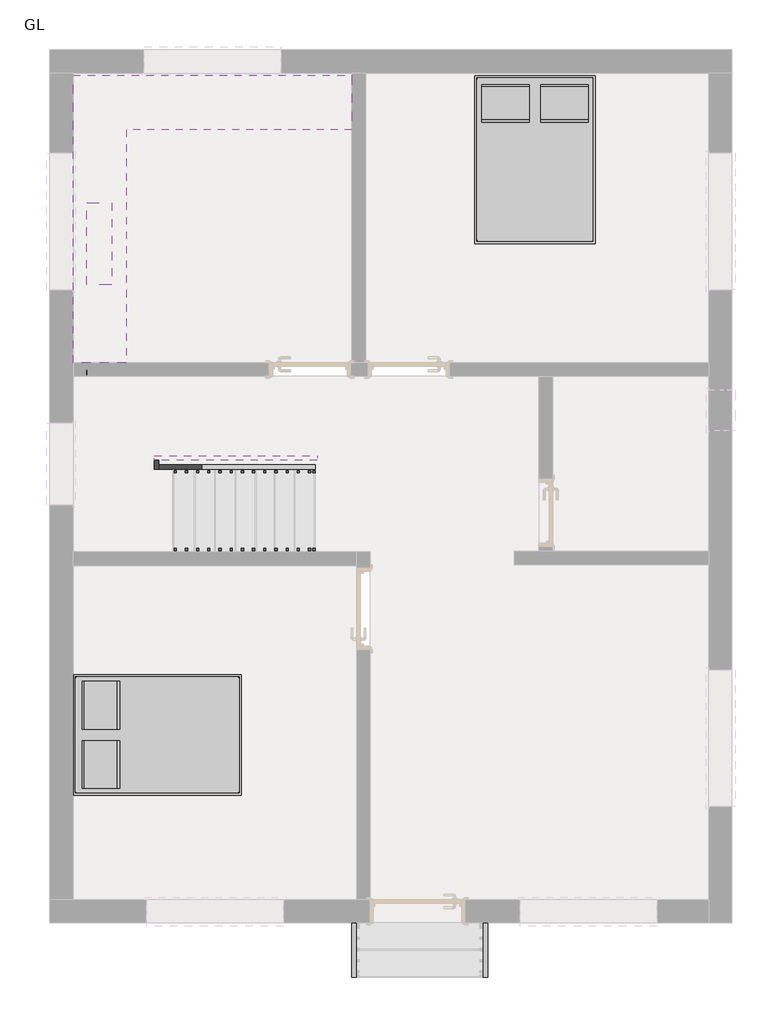
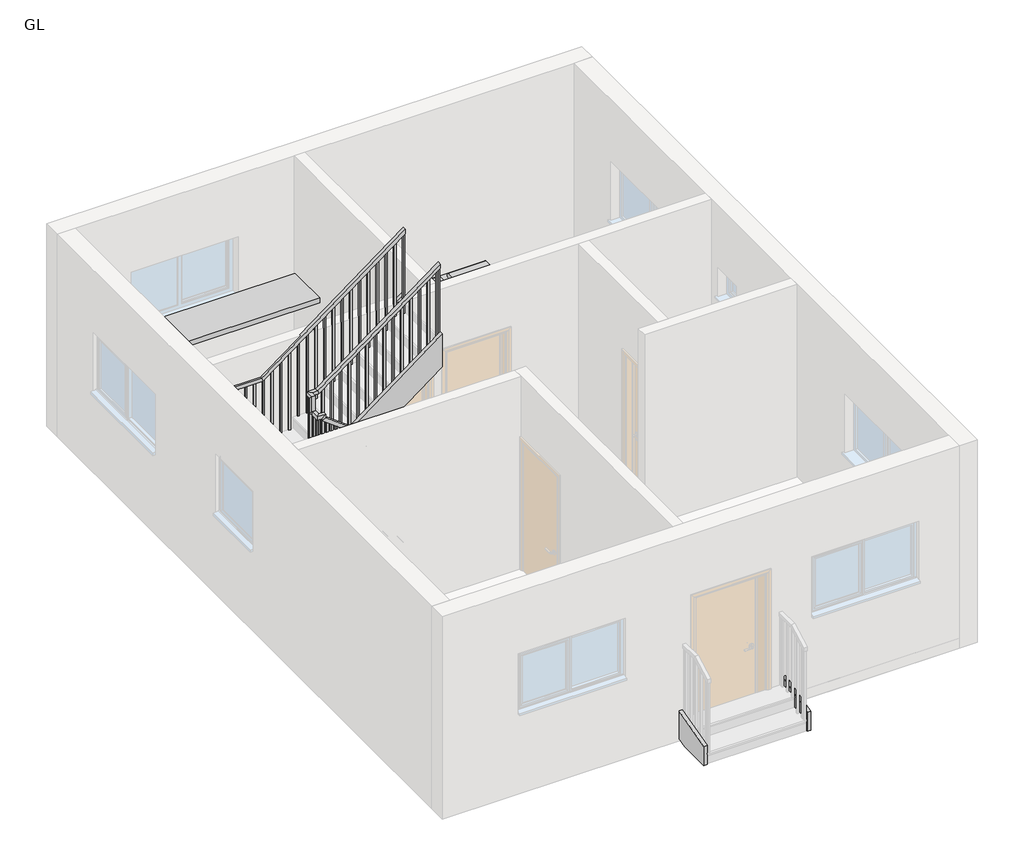
# One storey, part 2 of 2: 8 members, 2 furniture elements, 2 proxies, 2 railings.
"""IFC4 building model written with IfcOpenShell, lengths in millimetres."""

from ifc_helpers import new_model, si_unit, frame, origin, place, context, project, spatial, polyline, outline, extrude, faceted_brep, transform, mapped, element, save
from components import generic_models_1_generic_models_1_ec2a76fc, generic_models_2_generic_models_2_056d5301, furniture_bed_1_1346x1880x355mm_double_93dec6ea

model = new_model("IFC4")

# Units and contexts
model_context = context("Model", 3, world=origin())
ifc_project = project(units=[si_unit("LENGTHUNIT", "METRE", prefix="MILLI")], contexts=[model_context])

# Site, building, storey
site = spatial("IfcSite", under=ifc_project)
building = spatial("IfcBuilding", under=site)
storey = spatial("IfcBuildingStorey", under=building, Name="GL", Elevation=0.0)

# Proxies
placement = place(None, origin())
generic_models_1_generic_models_1_shape = generic_models_1_generic_models_1_ec2a76fc(model_context)
element("IfcBuildingElementProxy", 1, Name="Generic Models 1 : Generic Models 1", ObjectType="Generic Models 1 : Generic Models 1", at=placement, inside=storey, context=model_context, shape_type="MappedRepresentation", body=[
    mapped(generic_models_1_generic_models_1_shape, transform((0.0, 0.0, 0.0), x_axis=(1.0, 0.0, 0.0), y_axis=(0.0, 1.0, 0.0), z_axis=(0.0, 0.0, 1.0))),
])
generic_models_2_generic_models_2_shape = generic_models_2_generic_models_2_056d5301(model_context)
element("IfcBuildingElementProxy", 2, Name="Generic Models 2 : Generic Models 2", ObjectType="Generic Models 2 : Generic Models 2", at=placement, inside=storey, context=model_context, shape_type="MappedRepresentation", body=[
    mapped(generic_models_2_generic_models_2_shape, transform((0.0, 0.0, 0.0), x_axis=(1.0, 0.0, 0.0), y_axis=(0.0, 1.0, 0.0), z_axis=(0.0, 0.0, 1.0))),
])

# Furniture
furniture_bed_1_1346x1880x355mm_double_shape = furniture_bed_1_1346x1880x355mm_double_93dec6ea(model_context)
element("IfcFurniture", 3, ObjectType="Furniture_Bed_1 : 1346x1880x355mm-Double", at=placement, inside=storey, context=model_context, shape_type="MappedRepresentation", body=[
    mapped(furniture_bed_1_1346x1880x355mm_double_shape, transform((6044.9756135, 10437.9267123, 149.9616), x_axis=(1.0, 0.0, 0.0), y_axis=(0.0, 1.0, 0.0), z_axis=(0.0, 0.0, 1.0))),
])
element("IfcFurniture", 4, ObjectType="Furniture_Bed_1 : 1346x1880x355mm-Double", at=placement, inside=storey, context=model_context, shape_type="MappedRepresentation", body=[
    mapped(furniture_bed_1_1346x1880x355mm_double_shape, transform((1929.3384143, 3437.1747451, 149.9616), x_axis=(0.0, 1.0, 0.0), y_axis=(-1.0, 0.0, 0.0), z_axis=(0.0, 0.0, 1.0))),
])

# Members
element("IfcMember", 5, ObjectType="Stringer-50mm_Width", at=placement, inside=storey, context=model_context, shape_type="SweptSolid", body=[
    extrude(outline(polyline([(0.0, 3927.9747157), (240.3799463, 3927.9747157), (1566.4365081, 2174.3169781), (1566.4365081, 1511.1244088), (0.0, 3582.6751873), (0.0, 3927.9747157)])), frame((0.0, 5770.9272041, 0.0), z_axis=(0.0, 1.0, 0.0), x_axis=(0.0, 0.0, 1.0)), (0.0, 0.0, 1.0), 50.0),
])
element("IfcMember", 6, ObjectType="Stringer-50mm_Width", at=placement, inside=storey, context=model_context, shape_type="SweptSolid", body=[
    extrude(outline(polyline([(1223.7679225, 5770.9272041), (1173.7679225, 5770.9272041), (1173.7679225, 7802.1353898), (1223.7679225, 7802.1353898), (1223.7679225, 5770.9272041)])), frame((0.0, 0.0, 1166.4365081), z_axis=(0.0, 0.0, 1.0), x_axis=(1.0, 0.0, 0.0)), (0.0, 0.0, 1.0), 400.0),
])
element("IfcMember", 7, ObjectType="Stringer-50mm_Width", at=placement, inside=storey, context=model_context, shape_type="SweptSolid", body=[
    extrude(outline(polyline([(1166.4365081, 1997.5960405), (2630.7773804, 3949.8187157), (3130.7987558, 3949.8187157), (1166.4365081, 1330.9800323), (1166.4365081, 1997.5960405)])), frame((0.0, 7802.1353898, 0.0), z_axis=(0.0, 1.0, 0.0), x_axis=(0.0, 0.0, 1.0)), (0.0, 0.0, 1.0), 50.0),
])
element("IfcMember", 8, ObjectType="Stringer-50mm_Width", at=placement, inside=storey, context=model_context, shape_type="SweptSolid", body=[
    extrude(outline(polyline([(0.0, 3927.9747157), (240.3799463, 3927.9747157), (1560.7645481, 2181.8179225), (1059.2807982, 2181.8179225), (0.0, 3582.6751873), (0.0, 3927.9747157)])), frame((0.0, 6741.6853898, 0.0), z_axis=(0.0, 1.0, 0.0), x_axis=(0.0, 0.0, 1.0)), (0.0, 0.0, 1.0), 50.0),
])
element("IfcMember", 9, ObjectType="Stringer-50mm_Width", at=placement, inside=storey, context=model_context, shape_type="SweptSolid", body=[
    extrude(outline(polyline([(2181.8179225, 6741.6853898), (2131.8179225, 6741.6853898), (2131.8179225, 6844.0853898), (2181.8179225, 6844.0853898), (2181.8179225, 6741.6853898)])), frame((0.0, 0.0, 1166.4365081), z_axis=(0.0, 0.0, 1.0), x_axis=(1.0, 0.0, 0.0)), (0.0, 0.0, 1.0), 400.0),
])
element("IfcMember", 10, ObjectType="Stringer-50mm_Width", at=placement, inside=storey, context=model_context, shape_type="SweptSolid", body=[
    extrude(outline(polyline([(1767.1362488, 2131.8179225), (1267.1148735, 2131.8179225), (2630.7773804, 3949.8187157), (3130.7987558, 3949.8187157), (1767.1362488, 2131.8179225)])), frame((0.0, 6844.0853898, 0.0), z_axis=(0.0, 1.0, 0.0), x_axis=(0.0, 0.0, 1.0)), (0.0, 0.0, 1.0), 50.0),
])
element("IfcMember", 11, ObjectType="Stringer-50mm_Width", at=placement, inside=storey, context=model_context, shape_type="SweptSolid", body=[
    extrude(outline(polyline([(1066.0472041, 0.0), (1066.0472041, 285.8067966), (1675.6472041, 455.14013), (1675.6472041, 39.994759), (1531.6660715, 0.0), (1066.0472041, 0.0)])), frame((4335.1747157, 0.0, 0.0), z_axis=(1.0, 0.0, 0.0), x_axis=(0.0, 1.0, 0.0)), (0.0, 0.0, 1.0), 50.0),
])
element("IfcMember", 12, ObjectType="Stringer-50mm_Width", at=placement, inside=storey, context=model_context, shape_type="SweptSolid", body=[
    extrude(outline(polyline([(1066.0472041, 0.0), (1066.0472041, 285.8067966), (1675.6472041, 455.14013), (1675.6472041, 39.994759), (1531.6660715, 0.0), (1066.0472041, 0.0)])), frame((5807.5747157, 0.0, 0.0), z_axis=(1.0, 0.0, 0.0), x_axis=(0.0, 1.0, 0.0)), (0.0, 0.0, 1.0), 50.0),
])

# Railings
element("IfcRailing", 13, ObjectType="1100mm", at=placement, inside=storey, context=model_context, shape_type="SolidModel", body=[
    faceted_brep([(3927.9747157, 6691.2853898, 1269.3333333), (3927.9747157, 6691.2853898, 1206.7070206), (3927.9747157, 6741.2853898, 1206.7070206), (3927.9747157, 6741.2853898, 1269.3333333), (2206.4179225, 6691.2853898, 2567.7364635), (2156.4179225, 6691.2853898, 2542.8202959), (2156.4179225, 6741.2853898, 2542.8202959), (2206.4179225, 6741.2853898, 2567.7364635), (2206.4179225, 6691.2853898, 2624.0), (2156.4179225, 6691.2853898, 2574.0), (2156.4179225, 6741.2853898, 2574.0), (2206.4179225, 6741.2853898, 2624.0), (2081.4179225, 6691.2853898, 2624.0), (2081.4179225, 6691.2853898, 2574.0), (2131.4179225, 6741.2853898, 2574.0), (2131.4179225, 6741.2853898, 2624.0), (2081.4179225, 6816.2853898, 2624.0), (2081.4179225, 6816.2853898, 2574.0), (2131.4179225, 6816.2853898, 2574.0), (2131.4179225, 6816.2853898, 2624.0), (2081.4179225, 6819.4853898, 2624.0), (2081.4179225, 6869.4853898, 2574.0), (2131.4179225, 6869.4853898, 2574.0), (2131.4179225, 6819.4853898, 2624.0), (2081.4179225, 6819.4853898, 2848.9208412), (2081.4179225, 6869.4853898, 2798.9208412), (2131.4179225, 6869.4853898, 2798.9208412), (2131.4179225, 6819.4853898, 2848.9208412), (2081.4179225, 6944.4853898, 2848.9208412), (2081.4179225, 6944.4853898, 2798.9208412), (2131.4179225, 6894.4853898, 2798.9208412), (2131.4179225, 6894.4853898, 2848.9208412), (2206.4179225, 6944.4853898, 2848.9208412), (2222.9980476, 6944.4853898, 2798.9208412), (2222.9980476, 6894.4853898, 2798.9208412), (2206.4179225, 6894.4853898, 2848.9208412), (3949.8187157, 6944.4853898, 4148.0), (3949.8187157, 6894.4853898, 4148.0), (3949.8187157, 6894.4853898, 4085.6454714), (3949.8187157, 6944.4853898, 4085.6454714)], [[[0, 1, 2, 3]], [[1, 0, 4, 5]], [[2, 1, 5, 6]], [[3, 2, 6, 7]], [[0, 3, 7, 4]], [[5, 4, 8, 9]], [[6, 5, 9, 10]], [[7, 6, 10, 11]], [[4, 7, 11, 8]], [[9, 8, 12, 13]], [[10, 9, 13, 14]], [[11, 10, 14, 15]], [[8, 11, 15, 12]], [[13, 12, 16, 17]], [[14, 13, 17, 18]], [[15, 14, 18, 19]], [[12, 15, 19, 16]], [[17, 16, 20, 21]], [[18, 17, 21, 22]], [[19, 18, 22, 23]], [[16, 19, 23, 20]], [[21, 20, 24, 25]], [[22, 21, 25, 26]], [[23, 22, 26, 27]], [[20, 23, 27, 24]], [[25, 24, 28, 29]], [[26, 25, 29, 30]], [[27, 26, 30, 31]], [[24, 27, 31, 28]], [[29, 28, 32, 33]], [[30, 29, 33, 34]], [[31, 30, 34, 35]], [[28, 31, 35, 32]], [[36, 37, 38, 39]], [[33, 32, 36, 39]], [[34, 33, 39, 38]], [[35, 34, 38, 37]], [[32, 35, 37, 36]]]),
    extrude(outline(polyline([(4053.3057673, 3906.4179225), (2878.6666667, 3906.4179225), (2878.6666667, 3931.4179225), (4071.9342886, 3931.4179225), (4053.3057673, 3906.4179225)])), frame((0.0, 6906.9853898, 0.0), z_axis=(0.0, 1.0, 0.0), x_axis=(0.0, 0.0, 1.0)), (0.0, 0.0, 1.0), 25.0),
    extrude(outline(polyline([(3960.1631603, 3781.4179225), (2878.6666667, 3781.4179225), (2878.6666667, 3806.4179225), (3978.7916817, 3806.4179225), (3960.1631603, 3781.4179225)])), frame((0.0, 6906.9853898, 0.0), z_axis=(0.0, 1.0, 0.0), x_axis=(0.0, 0.0, 1.0)), (0.0, 0.0, 1.0), 25.0),
    extrude(outline(polyline([(3867.0205533, 3656.4179225), (2709.3333333, 3656.4179225), (2709.3333333, 3681.4179225), (3885.6490747, 3681.4179225), (3867.0205533, 3656.4179225)])), frame((0.0, 6906.9853898, 0.0), z_axis=(0.0, 1.0, 0.0), x_axis=(0.0, 0.0, 1.0)), (0.0, 0.0, 1.0), 25.0),
    extrude(outline(polyline([(3773.8779464, 3531.4179225), (2709.3333333, 3531.4179225), (2709.3333333, 3556.4179225), (3792.5064678, 3556.4179225), (3773.8779464, 3531.4179225)])), frame((0.0, 6906.9853898, 0.0), z_axis=(0.0, 1.0, 0.0), x_axis=(0.0, 0.0, 1.0)), (0.0, 0.0, 1.0), 25.0),
    extrude(outline(polyline([(3680.7353394, 3406.4179225), (2540.0, 3406.4179225), (2540.0, 3431.4179225), (3699.3638608, 3431.4179225), (3680.7353394, 3406.4179225)])), frame((0.0, 6906.9853898, 0.0), z_axis=(0.0, 1.0, 0.0), x_axis=(0.0, 0.0, 1.0)), (0.0, 0.0, 1.0), 25.0),
    extrude(outline(polyline([(3587.5927324, 3281.4179225), (2540.0, 3281.4179225), (2540.0, 3306.4179225), (3606.2212538, 3306.4179225), (3587.5927324, 3281.4179225)])), frame((0.0, 6906.9853898, 0.0), z_axis=(0.0, 1.0, 0.0), x_axis=(0.0, 0.0, 1.0)), (0.0, 0.0, 1.0), 25.0),
    extrude(outline(polyline([(3494.4501255, 3156.4179225), (2370.6666667, 3156.4179225), (2370.6666667, 3181.4179225), (3513.0786469, 3181.4179225), (3494.4501255, 3156.4179225)])), frame((0.0, 6906.9853898, 0.0), z_axis=(0.0, 1.0, 0.0), x_axis=(0.0, 0.0, 1.0)), (0.0, 0.0, 1.0), 25.0),
    extrude(outline(polyline([(3401.3075185, 3031.4179225), (2370.6666667, 3031.4179225), (2370.6666667, 3056.4179225), (3419.9360399, 3056.4179225), (3401.3075185, 3031.4179225)])), frame((0.0, 6906.9853898, 0.0), z_axis=(0.0, 1.0, 0.0), x_axis=(0.0, 0.0, 1.0)), (0.0, 0.0, 1.0), 25.0),
    extrude(outline(polyline([(3308.1649116, 2906.4179225), (2201.3333333, 2906.4179225), (2201.3333333, 2931.4179225), (3326.7934329, 2931.4179225), (3308.1649116, 2906.4179225)])), frame((0.0, 6906.9853898, 0.0), z_axis=(0.0, 1.0, 0.0), x_axis=(0.0, 0.0, 1.0)), (0.0, 0.0, 1.0), 25.0),
    extrude(outline(polyline([(3215.0223046, 2781.4179225), (2032.0, 2781.4179225), (2032.0, 2806.4179225), (3233.650826, 2806.4179225), (3215.0223046, 2781.4179225)])), frame((0.0, 6906.9853898, 0.0), z_axis=(0.0, 1.0, 0.0), x_axis=(0.0, 0.0, 1.0)), (0.0, 0.0, 1.0), 25.0),
    extrude(outline(polyline([(3121.8796976, 2656.4179225), (2032.0, 2656.4179225), (2032.0, 2681.4179225), (3140.508219, 2681.4179225), (3121.8796976, 2656.4179225)])), frame((0.0, 6906.9853898, 0.0), z_axis=(0.0, 1.0, 0.0), x_axis=(0.0, 0.0, 1.0)), (0.0, 0.0, 1.0), 25.0),
    extrude(outline(polyline([(3028.7370907, 2531.4179225), (1862.6666667, 2531.4179225), (1862.6666667, 2556.4179225), (3047.3656121, 2556.4179225), (3028.7370907, 2531.4179225)])), frame((0.0, 6906.9853898, 0.0), z_axis=(0.0, 1.0, 0.0), x_axis=(0.0, 0.0, 1.0)), (0.0, 0.0, 1.0), 25.0),
    extrude(outline(polyline([(2935.5944837, 2406.4179225), (1862.6666667, 2406.4179225), (1862.6666667, 2431.4179225), (2954.2230051, 2431.4179225), (2935.5944837, 2406.4179225)])), frame((0.0, 6906.9853898, 0.0), z_axis=(0.0, 1.0, 0.0), x_axis=(0.0, 0.0, 1.0)), (0.0, 0.0, 1.0), 25.0),
    extrude(outline(polyline([(2842.4518767, 2281.4179225), (1693.3333333, 2281.4179225), (1693.3333333, 2306.4179225), (2861.0803981, 2306.4179225), (2842.4518767, 2281.4179225)])), frame((0.0, 6906.9853898, 0.0), z_axis=(0.0, 1.0, 0.0), x_axis=(0.0, 0.0, 1.0)), (0.0, 0.0, 1.0), 25.0),
    extrude(outline(polyline([(2156.4179225, 6906.9853898), (2156.4179225, 6931.9853898), (2181.4179225, 6931.9853898), (2181.4179225, 6906.9853898), (2156.4179225, 6906.9853898)])), frame((0.0, 0.0, 1693.3333333), z_axis=(0.0, 0.0, 1.0), x_axis=(1.0, 0.0, 0.0)), (0.0, 0.0, 1.0), 1105.5875078),
    extrude(outline(polyline([(2118.9179225, 6891.2853898), (2093.9179225, 6891.2853898), (2093.9179225, 6916.2853898), (2118.9179225, 6916.2853898), (2118.9179225, 6891.2853898)])), frame((0.0, 0.0, 1524.0), z_axis=(0.0, 0.0, 1.0), x_axis=(1.0, 0.0, 0.0)), (0.0, 0.0, 1.0), 1274.9208412),
    extrude(outline(polyline([(2118.9179225, 6766.2853898), (2093.9179225, 6766.2853898), (2093.9179225, 6791.2853898), (2118.9179225, 6791.2853898), (2118.9179225, 6766.2853898)])), frame((0.0, 0.0, 1524.0), z_axis=(0.0, 0.0, 1.0), x_axis=(1.0, 0.0, 0.0)), (0.0, 0.0, 1.0), 1050.0),
    extrude(outline(polyline([(2127.9747157, 6728.7853898), (2127.9747157, 6703.7853898), (2102.9747157, 6703.7853898), (2102.9747157, 6728.7853898), (2127.9747157, 6728.7853898)])), frame((0.0, 0.0, 1524.0), z_axis=(0.0, 0.0, 1.0), x_axis=(1.0, 0.0, 0.0)), (0.0, 0.0, 1.0), 1050.0),
    extrude(outline(polyline([(1354.6666667, 2252.9747157), (2469.9968822, 2252.9747157), (2488.8519548, 2227.9747157), (1354.6666667, 2227.9747157), (1354.6666667, 2252.9747157)])), frame((0.0, 6703.7853898, 0.0), z_axis=(0.0, 1.0, 0.0), x_axis=(0.0, 0.0, 1.0)), (0.0, 0.0, 1.0), 25.0),
    extrude(outline(polyline([(1185.3333333, 2377.9747157), (2375.7215194, 2377.9747157), (2394.576592, 2352.9747157), (1185.3333333, 2352.9747157), (1185.3333333, 2377.9747157)])), frame((0.0, 6703.7853898, 0.0), z_axis=(0.0, 1.0, 0.0), x_axis=(0.0, 0.0, 1.0)), (0.0, 0.0, 1.0), 25.0),
    extrude(outline(polyline([(1185.3333333, 2502.9747157), (2281.4461566, 2502.9747157), (2300.3012292, 2477.9747157), (1185.3333333, 2477.9747157), (1185.3333333, 2502.9747157)])), frame((0.0, 6703.7853898, 0.0), z_axis=(0.0, 1.0, 0.0), x_axis=(0.0, 0.0, 1.0)), (0.0, 0.0, 1.0), 25.0),
    extrude(outline(polyline([(1016.0, 2627.9747157), (2187.1707938, 2627.9747157), (2206.0258664, 2602.9747157), (1016.0, 2602.9747157), (1016.0, 2627.9747157)])), frame((0.0, 6703.7853898, 0.0), z_axis=(0.0, 1.0, 0.0), x_axis=(0.0, 0.0, 1.0)), (0.0, 0.0, 1.0), 25.0),
    extrude(outline(polyline([(1016.0, 2752.9747157), (2092.895431, 2752.9747157), (2111.7505036, 2727.9747157), (1016.0, 2727.9747157), (1016.0, 2752.9747157)])), frame((0.0, 6703.7853898, 0.0), z_axis=(0.0, 1.0, 0.0), x_axis=(0.0, 0.0, 1.0)), (0.0, 0.0, 1.0), 25.0),
    extrude(outline(polyline([(846.6666667, 2877.9747157), (1998.6200682, 2877.9747157), (2017.4751408, 2852.9747157), (846.6666667, 2852.9747157), (846.6666667, 2877.9747157)])), frame((0.0, 6703.7853898, 0.0), z_axis=(0.0, 1.0, 0.0), x_axis=(0.0, 0.0, 1.0)), (0.0, 0.0, 1.0), 25.0),
    extrude(outline(polyline([(846.6666667, 3002.9747157), (1904.3447054, 3002.9747157), (1923.1997779, 2977.9747157), (846.6666667, 2977.9747157), (846.6666667, 3002.9747157)])), frame((0.0, 6703.7853898, 0.0), z_axis=(0.0, 1.0, 0.0), x_axis=(0.0, 0.0, 1.0)), (0.0, 0.0, 1.0), 25.0),
    extrude(outline(polyline([(677.3333333, 3127.9747157), (1810.0693426, 3127.9747157), (1828.9244151, 3102.9747157), (677.3333333, 3102.9747157), (677.3333333, 3127.9747157)])), frame((0.0, 6703.7853898, 0.0), z_axis=(0.0, 1.0, 0.0), x_axis=(0.0, 0.0, 1.0)), (0.0, 0.0, 1.0), 25.0),
    extrude(outline(polyline([(677.3333333, 3252.9747157), (1715.7939798, 3252.9747157), (1734.6490523, 3227.9747157), (677.3333333, 3227.9747157), (677.3333333, 3252.9747157)])), frame((0.0, 6703.7853898, 0.0), z_axis=(0.0, 1.0, 0.0), x_axis=(0.0, 0.0, 1.0)), (0.0, 0.0, 1.0), 25.0),
    extrude(outline(polyline([(508.0, 3377.9747157), (1621.518617, 3377.9747157), (1640.3736895, 3352.9747157), (508.0, 3352.9747157), (508.0, 3377.9747157)])), frame((0.0, 6703.7853898, 0.0), z_axis=(0.0, 1.0, 0.0), x_axis=(0.0, 0.0, 1.0)), (0.0, 0.0, 1.0), 25.0),
    extrude(outline(polyline([(338.6666667, 3502.9747157), (1527.2432542, 3502.9747157), (1546.0983267, 3477.9747157), (338.6666667, 3477.9747157), (338.6666667, 3502.9747157)])), frame((0.0, 6703.7853898, 0.0), z_axis=(0.0, 1.0, 0.0), x_axis=(0.0, 0.0, 1.0)), (0.0, 0.0, 1.0), 25.0),
    extrude(outline(polyline([(338.6666667, 3627.9747157), (1432.9678913, 3627.9747157), (1451.8229639, 3602.9747157), (338.6666667, 3602.9747157), (338.6666667, 3627.9747157)])), frame((0.0, 6703.7853898, 0.0), z_axis=(0.0, 1.0, 0.0), x_axis=(0.0, 0.0, 1.0)), (0.0, 0.0, 1.0), 25.0),
    extrude(outline(polyline([(169.3333333, 3752.9747157), (1338.6925285, 3752.9747157), (1357.5476011, 3727.9747157), (169.3333333, 3727.9747157), (169.3333333, 3752.9747157)])), frame((0.0, 6703.7853898, 0.0), z_axis=(0.0, 1.0, 0.0), x_axis=(0.0, 0.0, 1.0)), (0.0, 0.0, 1.0), 25.0),
    extrude(outline(polyline([(169.3333333, 3877.9747157), (1244.4171657, 3877.9747157), (1263.2722383, 3852.9747157), (169.3333333, 3852.9747157), (169.3333333, 3877.9747157)])), frame((0.0, 6703.7853898, 0.0), z_axis=(0.0, 1.0, 0.0), x_axis=(0.0, 0.0, 1.0)), (0.0, 0.0, 1.0), 25.0),
    extrude(outline(polyline([(2118.9179225, 6906.9853898), (2093.9179225, 6906.9853898), (2093.9179225, 6931.9853898), (2118.9179225, 6931.9853898), (2118.9179225, 6906.9853898)])), frame((0.0, 0.0, 1524.0), z_axis=(0.0, 0.0, 1.0), x_axis=(1.0, 0.0, 0.0)), (0.0, 0.0, 1.0), 1274.9208412),
    extrude(outline(polyline([(2118.9179225, 6728.7853898), (2118.9179225, 6703.7853898), (2093.9179225, 6703.7853898), (2093.9179225, 6728.7853898), (2118.9179225, 6728.7853898)])), frame((0.0, 0.0, 1524.0), z_axis=(0.0, 0.0, 1.0), x_axis=(1.0, 0.0, 0.0)), (0.0, 0.0, 1.0), 1050.0),
    extrude(outline(polyline([(4067.01695, 3924.8187157), (2878.6666667, 3924.8187157), (2878.6666667, 3949.8187157), (4085.6454714, 3949.8187157), (4067.01695, 3924.8187157)])), frame((0.0, 6906.9853898, 0.0), z_axis=(0.0, 1.0, 0.0), x_axis=(0.0, 0.0, 1.0)), (0.0, 0.0, 1.0), 25.0),
    extrude(outline(polyline([(169.3333333, 3927.9747157), (1206.7070206, 3927.9747157), (1225.5620932, 3902.9747157), (169.3333333, 3902.9747157), (169.3333333, 3927.9747157)])), frame((0.0, 6703.7853898, 0.0), z_axis=(0.0, 1.0, 0.0), x_axis=(0.0, 0.0, 1.0)), (0.0, 0.0, 1.0), 25.0),
])
element("IfcRailing", 14, ObjectType="1100mm", at=placement, inside=storey, context=model_context, shape_type="SolidModel", body=[
    faceted_brep([(3927.9747157, 5821.3272041, 1269.3333333), (3927.9747157, 5821.3272041, 1206.7070206), (3927.9747157, 5871.3272041, 1206.7070206), (3927.9747157, 5871.3272041, 1269.3333333), (2131.8179225, 5821.3272041, 2624.0), (2115.0766548, 5821.3272041, 2574.0), (2115.0766548, 5871.3272041, 2574.0), (2131.8179225, 5871.3272041, 2624.0), (1224.1679225, 5821.3272041, 2624.0), (1224.1679225, 5821.3272041, 2574.0), (1274.1679225, 5871.3272041, 2574.0), (1274.1679225, 5871.3272041, 2624.0), (1224.1679225, 7801.7353898, 2624.0), (1224.1679225, 7801.7353898, 2574.0), (1274.1679225, 7751.7353898, 2574.0), (1274.1679225, 7751.7353898, 2624.0), (1904.5678234, 7801.7353898, 2624.0), (1921.1479485, 7801.7353898, 2574.0), (1921.1479485, 7751.7353898, 2574.0), (1904.5678234, 7751.7353898, 2624.0), (3949.8187157, 7801.7353898, 4148.0), (3949.8187157, 7751.7353898, 4148.0), (3949.8187157, 7751.7353898, 4085.6454714), (3949.8187157, 7801.7353898, 4085.6454714)], [[[0, 1, 2, 3]], [[1, 0, 4, 5]], [[2, 1, 5, 6]], [[3, 2, 6, 7]], [[0, 3, 7, 4]], [[5, 4, 8, 9]], [[6, 5, 9, 10]], [[7, 6, 10, 11]], [[4, 7, 11, 8]], [[9, 8, 12, 13]], [[10, 9, 13, 14]], [[11, 10, 14, 15]], [[8, 11, 15, 12]], [[13, 12, 16, 17]], [[14, 13, 17, 18]], [[15, 14, 18, 19]], [[12, 15, 19, 16]], [[20, 21, 22, 23]], [[17, 16, 20, 23]], [[18, 17, 23, 22]], [[19, 18, 22, 21]], [[16, 19, 21, 20]]]),
    extrude(outline(polyline([(2878.6666667, 3924.1679225), (2878.6666667, 3949.1679225), (4085.3849718, 3949.1679225), (4066.539271, 3924.1679225), (2878.6666667, 3924.1679225)])), frame((0.0, 7764.2353898, 0.0), z_axis=(0.0, 1.0, 0.0), x_axis=(0.0, 0.0, 1.0)), (0.0, 0.0, 1.0), 25.0),
    extrude(outline(polyline([(2878.6666667, 3799.1679225), (2878.6666667, 3824.1679225), (3992.0179319, 3824.1679225), (3973.3894105, 3799.1679225), (2878.6666667, 3799.1679225)])), frame((0.0, 7764.2353898, 0.0), z_axis=(0.0, 1.0, 0.0), x_axis=(0.0, 0.0, 1.0)), (0.0, 0.0, 1.0), 25.0),
    extrude(outline(polyline([(2709.3333333, 3674.1679225), (2709.3333333, 3699.1679225), (3898.8753249, 3699.1679225), (3880.2468035, 3674.1679225), (2709.3333333, 3674.1679225)])), frame((0.0, 7764.2353898, 0.0), z_axis=(0.0, 1.0, 0.0), x_axis=(0.0, 0.0, 1.0)), (0.0, 0.0, 1.0), 25.0),
    extrude(outline(polyline([(2709.3333333, 3549.1679225), (2709.3333333, 3574.1679225), (3805.7327179, 3574.1679225), (3787.1041966, 3549.1679225), (2709.3333333, 3549.1679225)])), frame((0.0, 7764.2353898, 0.0), z_axis=(0.0, 1.0, 0.0), x_axis=(0.0, 0.0, 1.0)), (0.0, 0.0, 1.0), 25.0),
    extrude(outline(polyline([(2540.0, 3424.1679225), (2540.0, 3449.1679225), (3712.590111, 3449.1679225), (3693.9615896, 3424.1679225), (2540.0, 3424.1679225)])), frame((0.0, 7764.2353898, 0.0), z_axis=(0.0, 1.0, 0.0), x_axis=(0.0, 0.0, 1.0)), (0.0, 0.0, 1.0), 25.0),
    extrude(outline(polyline([(2540.0, 3299.1679225), (2540.0, 3324.1679225), (3619.447504, 3324.1679225), (3600.8189826, 3299.1679225), (2540.0, 3299.1679225)])), frame((0.0, 7764.2353898, 0.0), z_axis=(0.0, 1.0, 0.0), x_axis=(0.0, 0.0, 1.0)), (0.0, 0.0, 1.0), 25.0),
    extrude(outline(polyline([(2370.6666667, 3174.1679225), (2370.6666667, 3199.1679225), (3526.3048971, 3199.1679225), (3507.6763757, 3174.1679225), (2370.6666667, 3174.1679225)])), frame((0.0, 7764.2353898, 0.0), z_axis=(0.0, 1.0, 0.0), x_axis=(0.0, 0.0, 1.0)), (0.0, 0.0, 1.0), 25.0),
    extrude(outline(polyline([(2370.6666667, 3049.1679225), (2370.6666667, 3074.1679225), (3433.1622901, 3074.1679225), (3414.5337687, 3049.1679225), (2370.6666667, 3049.1679225)])), frame((0.0, 7764.2353898, 0.0), z_axis=(0.0, 1.0, 0.0), x_axis=(0.0, 0.0, 1.0)), (0.0, 0.0, 1.0), 25.0),
    extrude(outline(polyline([(2201.3333333, 2924.1679225), (2201.3333333, 2949.1679225), (3340.0196831, 2949.1679225), (3321.3911617, 2924.1679225), (2201.3333333, 2924.1679225)])), frame((0.0, 7764.2353898, 0.0), z_axis=(0.0, 1.0, 0.0), x_axis=(0.0, 0.0, 1.0)), (0.0, 0.0, 1.0), 25.0),
    extrude(outline(polyline([(2201.3333333, 2799.1679225), (2201.3333333, 2824.1679225), (3246.8770762, 2824.1679225), (3228.2485548, 2799.1679225), (2201.3333333, 2799.1679225)])), frame((0.0, 7764.2353898, 0.0), z_axis=(0.0, 1.0, 0.0), x_axis=(0.0, 0.0, 1.0)), (0.0, 0.0, 1.0), 25.0),
    extrude(outline(polyline([(2032.0, 2674.1679225), (2032.0, 2699.1679225), (3153.7344692, 2699.1679225), (3135.1059478, 2674.1679225), (2032.0, 2674.1679225)])), frame((0.0, 7764.2353898, 0.0), z_axis=(0.0, 1.0, 0.0), x_axis=(0.0, 0.0, 1.0)), (0.0, 0.0, 1.0), 25.0),
    extrude(outline(polyline([(1862.6666667, 2549.1679225), (1862.6666667, 2574.1679225), (3060.5918622, 2574.1679225), (3041.9633409, 2549.1679225), (1862.6666667, 2549.1679225)])), frame((0.0, 7764.2353898, 0.0), z_axis=(0.0, 1.0, 0.0), x_axis=(0.0, 0.0, 1.0)), (0.0, 0.0, 1.0), 25.0),
    extrude(outline(polyline([(1862.6666667, 2424.1679225), (1862.6666667, 2449.1679225), (2967.4492553, 2449.1679225), (2948.8207339, 2424.1679225), (1862.6666667, 2424.1679225)])), frame((0.0, 7764.2353898, 0.0), z_axis=(0.0, 1.0, 0.0), x_axis=(0.0, 0.0, 1.0)), (0.0, 0.0, 1.0), 25.0),
    extrude(outline(polyline([(1693.3333333, 2299.1679225), (1693.3333333, 2324.1679225), (2874.3066483, 2324.1679225), (2855.6781269, 2299.1679225), (1693.3333333, 2299.1679225)])), frame((0.0, 7764.2353898, 0.0), z_axis=(0.0, 1.0, 0.0), x_axis=(0.0, 0.0, 1.0)), (0.0, 0.0, 1.0), 25.0),
    extrude(outline(polyline([(1693.3333333, 2174.1679225), (1693.3333333, 2199.1679225), (2781.1640414, 2199.1679225), (2762.53552, 2174.1679225), (1693.3333333, 2174.1679225)])), frame((0.0, 7764.2353898, 0.0), z_axis=(0.0, 1.0, 0.0), x_axis=(0.0, 0.0, 1.0)), (0.0, 0.0, 1.0), 25.0),
    extrude(outline(polyline([(1524.0, 2049.1679225), (1524.0, 2074.1679225), (2688.0214344, 2074.1679225), (2669.392913, 2049.1679225), (1524.0, 2049.1679225)])), frame((0.0, 7764.2353898, 0.0), z_axis=(0.0, 1.0, 0.0), x_axis=(0.0, 0.0, 1.0)), (0.0, 0.0, 1.0), 25.0),
    extrude(outline(polyline([(1524.0, 1924.1679225), (1524.0, 1949.1679225), (2594.8788274, 1949.1679225), (2576.250306, 1924.1679225), (1524.0, 1924.1679225)])), frame((0.0, 7764.2353898, 0.0), z_axis=(0.0, 1.0, 0.0), x_axis=(0.0, 0.0, 1.0)), (0.0, 0.0, 1.0), 25.0),
    extrude(outline(polyline([(1799.1679225, 7789.2353898), (1824.1679225, 7789.2353898), (1824.1679225, 7764.2353898), (1799.1679225, 7764.2353898), (1799.1679225, 7789.2353898)])), frame((0.0, 0.0, 1524.0), z_axis=(0.0, 0.0, 1.0), x_axis=(1.0, 0.0, 0.0)), (0.0, 0.0, 1.0), 1050.0),
    extrude(outline(polyline([(1674.1679225, 7789.2353898), (1699.1679225, 7789.2353898), (1699.1679225, 7764.2353898), (1674.1679225, 7764.2353898), (1674.1679225, 7789.2353898)])), frame((0.0, 0.0, 1524.0), z_axis=(0.0, 0.0, 1.0), x_axis=(1.0, 0.0, 0.0)), (0.0, 0.0, 1.0), 1050.0),
    extrude(outline(polyline([(1549.1679225, 7789.2353898), (1574.1679225, 7789.2353898), (1574.1679225, 7764.2353898), (1549.1679225, 7764.2353898), (1549.1679225, 7789.2353898)])), frame((0.0, 0.0, 1524.0), z_axis=(0.0, 0.0, 1.0), x_axis=(1.0, 0.0, 0.0)), (0.0, 0.0, 1.0), 1050.0),
    extrude(outline(polyline([(1424.1679225, 7789.2353898), (1449.1679225, 7789.2353898), (1449.1679225, 7764.2353898), (1424.1679225, 7764.2353898), (1424.1679225, 7789.2353898)])), frame((0.0, 0.0, 1524.0), z_axis=(0.0, 0.0, 1.0), x_axis=(1.0, 0.0, 0.0)), (0.0, 0.0, 1.0), 1050.0),
    extrude(outline(polyline([(1299.1679225, 7789.2353898), (1324.1679225, 7789.2353898), (1324.1679225, 7764.2353898), (1299.1679225, 7764.2353898), (1299.1679225, 7789.2353898)])), frame((0.0, 0.0, 1524.0), z_axis=(0.0, 0.0, 1.0), x_axis=(1.0, 0.0, 0.0)), (0.0, 0.0, 1.0), 1050.0),
    extrude(outline(polyline([(1236.6679225, 7646.3272041), (1236.6679225, 7671.3272041), (1261.6679225, 7671.3272041), (1261.6679225, 7646.3272041), (1236.6679225, 7646.3272041)])), frame((0.0, 0.0, 1524.0), z_axis=(0.0, 0.0, 1.0), x_axis=(1.0, 0.0, 0.0)), (0.0, 0.0, 1.0), 1050.0),
    extrude(outline(polyline([(1236.6679225, 7521.3272041), (1236.6679225, 7546.3272041), (1261.6679225, 7546.3272041), (1261.6679225, 7521.3272041), (1236.6679225, 7521.3272041)])), frame((0.0, 0.0, 1524.0), z_axis=(0.0, 0.0, 1.0), x_axis=(1.0, 0.0, 0.0)), (0.0, 0.0, 1.0), 1050.0),
    extrude(outline(polyline([(1236.6679225, 7396.3272041), (1236.6679225, 7421.3272041), (1261.6679225, 7421.3272041), (1261.6679225, 7396.3272041), (1236.6679225, 7396.3272041)])), frame((0.0, 0.0, 1524.0), z_axis=(0.0, 0.0, 1.0), x_axis=(1.0, 0.0, 0.0)), (0.0, 0.0, 1.0), 1050.0),
    extrude(outline(polyline([(1236.6679225, 7271.3272041), (1236.6679225, 7296.3272041), (1261.6679225, 7296.3272041), (1261.6679225, 7271.3272041), (1236.6679225, 7271.3272041)])), frame((0.0, 0.0, 1524.0), z_axis=(0.0, 0.0, 1.0), x_axis=(1.0, 0.0, 0.0)), (0.0, 0.0, 1.0), 1050.0),
    extrude(outline(polyline([(1236.6679225, 7146.3272041), (1236.6679225, 7171.3272041), (1261.6679225, 7171.3272041), (1261.6679225, 7146.3272041), (1236.6679225, 7146.3272041)])), frame((0.0, 0.0, 1524.0), z_axis=(0.0, 0.0, 1.0), x_axis=(1.0, 0.0, 0.0)), (0.0, 0.0, 1.0), 1050.0),
    extrude(outline(polyline([(1236.6679225, 7021.3272041), (1236.6679225, 7046.3272041), (1261.6679225, 7046.3272041), (1261.6679225, 7021.3272041), (1236.6679225, 7021.3272041)])), frame((0.0, 0.0, 1524.0), z_axis=(0.0, 0.0, 1.0), x_axis=(1.0, 0.0, 0.0)), (0.0, 0.0, 1.0), 1050.0),
    extrude(outline(polyline([(1236.6679225, 6896.3272041), (1236.6679225, 6921.3272041), (1261.6679225, 6921.3272041), (1261.6679225, 6896.3272041), (1236.6679225, 6896.3272041)])), frame((0.0, 0.0, 1524.0), z_axis=(0.0, 0.0, 1.0), x_axis=(1.0, 0.0, 0.0)), (0.0, 0.0, 1.0), 1050.0),
    extrude(outline(polyline([(1236.6679225, 6771.3272041), (1236.6679225, 6796.3272041), (1261.6679225, 6796.3272041), (1261.6679225, 6771.3272041), (1236.6679225, 6771.3272041)])), frame((0.0, 0.0, 1524.0), z_axis=(0.0, 0.0, 1.0), x_axis=(1.0, 0.0, 0.0)), (0.0, 0.0, 1.0), 1050.0),
    extrude(outline(polyline([(1236.6679225, 6646.3272041), (1236.6679225, 6671.3272041), (1261.6679225, 6671.3272041), (1261.6679225, 6646.3272041), (1236.6679225, 6646.3272041)])), frame((0.0, 0.0, 1524.0), z_axis=(0.0, 0.0, 1.0), x_axis=(1.0, 0.0, 0.0)), (0.0, 0.0, 1.0), 1050.0),
    extrude(outline(polyline([(1236.6679225, 6521.3272041), (1236.6679225, 6546.3272041), (1261.6679225, 6546.3272041), (1261.6679225, 6521.3272041), (1236.6679225, 6521.3272041)])), frame((0.0, 0.0, 1524.0), z_axis=(0.0, 0.0, 1.0), x_axis=(1.0, 0.0, 0.0)), (0.0, 0.0, 1.0), 1050.0),
    extrude(outline(polyline([(1236.6679225, 6396.3272041), (1236.6679225, 6421.3272041), (1261.6679225, 6421.3272041), (1261.6679225, 6396.3272041), (1236.6679225, 6396.3272041)])), frame((0.0, 0.0, 1524.0), z_axis=(0.0, 0.0, 1.0), x_axis=(1.0, 0.0, 0.0)), (0.0, 0.0, 1.0), 1050.0),
    extrude(outline(polyline([(1236.6679225, 6271.3272041), (1236.6679225, 6296.3272041), (1261.6679225, 6296.3272041), (1261.6679225, 6271.3272041), (1236.6679225, 6271.3272041)])), frame((0.0, 0.0, 1524.0), z_axis=(0.0, 0.0, 1.0), x_axis=(1.0, 0.0, 0.0)), (0.0, 0.0, 1.0), 1050.0),
    extrude(outline(polyline([(1236.6679225, 6146.3272041), (1236.6679225, 6171.3272041), (1261.6679225, 6171.3272041), (1261.6679225, 6146.3272041), (1236.6679225, 6146.3272041)])), frame((0.0, 0.0, 1524.0), z_axis=(0.0, 0.0, 1.0), x_axis=(1.0, 0.0, 0.0)), (0.0, 0.0, 1.0), 1050.0),
    extrude(outline(polyline([(1236.6679225, 6021.3272041), (1236.6679225, 6046.3272041), (1261.6679225, 6046.3272041), (1261.6679225, 6021.3272041), (1236.6679225, 6021.3272041)])), frame((0.0, 0.0, 1524.0), z_axis=(0.0, 0.0, 1.0), x_axis=(1.0, 0.0, 0.0)), (0.0, 0.0, 1.0), 1050.0),
    extrude(outline(polyline([(1236.6679225, 5896.3272041), (1236.6679225, 5921.3272041), (1261.6679225, 5921.3272041), (1261.6679225, 5896.3272041), (1236.6679225, 5896.3272041)])), frame((0.0, 0.0, 1524.0), z_axis=(0.0, 0.0, 1.0), x_axis=(1.0, 0.0, 0.0)), (0.0, 0.0, 1.0), 1050.0),
    extrude(outline(polyline([(1377.9747157, 5833.8272041), (1352.9747157, 5833.8272041), (1352.9747157, 5858.8272041), (1377.9747157, 5858.8272041), (1377.9747157, 5833.8272041)])), frame((0.0, 0.0, 1524.0), z_axis=(0.0, 0.0, 1.0), x_axis=(1.0, 0.0, 0.0)), (0.0, 0.0, 1.0), 1050.0),
    extrude(outline(polyline([(1502.9747157, 5833.8272041), (1477.9747157, 5833.8272041), (1477.9747157, 5858.8272041), (1502.9747157, 5858.8272041), (1502.9747157, 5833.8272041)])), frame((0.0, 0.0, 1524.0), z_axis=(0.0, 0.0, 1.0), x_axis=(1.0, 0.0, 0.0)), (0.0, 0.0, 1.0), 1050.0),
    extrude(outline(polyline([(1627.9747157, 5833.8272041), (1602.9747157, 5833.8272041), (1602.9747157, 5858.8272041), (1627.9747157, 5858.8272041), (1627.9747157, 5833.8272041)])), frame((0.0, 0.0, 1524.0), z_axis=(0.0, 0.0, 1.0), x_axis=(1.0, 0.0, 0.0)), (0.0, 0.0, 1.0), 1050.0),
    extrude(outline(polyline([(1752.9747157, 5833.8272041), (1727.9747157, 5833.8272041), (1727.9747157, 5858.8272041), (1752.9747157, 5858.8272041), (1752.9747157, 5833.8272041)])), frame((0.0, 0.0, 1524.0), z_axis=(0.0, 0.0, 1.0), x_axis=(1.0, 0.0, 0.0)), (0.0, 0.0, 1.0), 1050.0),
    extrude(outline(polyline([(1877.9747157, 5833.8272041), (1852.9747157, 5833.8272041), (1852.9747157, 5858.8272041), (1877.9747157, 5858.8272041), (1877.9747157, 5833.8272041)])), frame((0.0, 0.0, 1524.0), z_axis=(0.0, 0.0, 1.0), x_axis=(1.0, 0.0, 0.0)), (0.0, 0.0, 1.0), 1050.0),
    extrude(outline(polyline([(2002.9747157, 5833.8272041), (1977.9747157, 5833.8272041), (1977.9747157, 5858.8272041), (2002.9747157, 5858.8272041), (2002.9747157, 5833.8272041)])), frame((0.0, 0.0, 1524.0), z_axis=(0.0, 0.0, 1.0), x_axis=(1.0, 0.0, 0.0)), (0.0, 0.0, 1.0), 1050.0),
    extrude(outline(polyline([(2127.9747157, 5833.8272041), (2102.9747157, 5833.8272041), (2102.9747157, 5858.8272041), (2127.9747157, 5858.8272041), (2127.9747157, 5833.8272041)])), frame((0.0, 0.0, 1524.0), z_axis=(0.0, 0.0, 1.0), x_axis=(1.0, 0.0, 0.0)), (0.0, 0.0, 1.0), 1050.0),
    extrude(outline(polyline([(2469.9968822, 2252.9747157), (2488.8519548, 2227.9747157), (1354.6666667, 2227.9747157), (1354.6666667, 2252.9747157), (2469.9968822, 2252.9747157)])), frame((0.0, 5833.8272041, 0.0), z_axis=(0.0, 1.0, 0.0), x_axis=(0.0, 0.0, 1.0)), (0.0, 0.0, 1.0), 25.0),
    extrude(outline(polyline([(2375.7215194, 2377.9747157), (2394.576592, 2352.9747157), (1185.3333333, 2352.9747157), (1185.3333333, 2377.9747157), (2375.7215194, 2377.9747157)])), frame((0.0, 5833.8272041, 0.0), z_axis=(0.0, 1.0, 0.0), x_axis=(0.0, 0.0, 1.0)), (0.0, 0.0, 1.0), 25.0),
    extrude(outline(polyline([(2281.4461566, 2502.9747157), (2300.3012292, 2477.9747157), (1185.3333333, 2477.9747157), (1185.3333333, 2502.9747157), (2281.4461566, 2502.9747157)])), frame((0.0, 5833.8272041, 0.0), z_axis=(0.0, 1.0, 0.0), x_axis=(0.0, 0.0, 1.0)), (0.0, 0.0, 1.0), 25.0),
    extrude(outline(polyline([(2187.1707938, 2627.9747157), (2206.0258664, 2602.9747157), (1016.0, 2602.9747157), (1016.0, 2627.9747157), (2187.1707938, 2627.9747157)])), frame((0.0, 5833.8272041, 0.0), z_axis=(0.0, 1.0, 0.0), x_axis=(0.0, 0.0, 1.0)), (0.0, 0.0, 1.0), 25.0),
    extrude(outline(polyline([(2092.895431, 2752.9747157), (2111.7505036, 2727.9747157), (1016.0, 2727.9747157), (1016.0, 2752.9747157), (2092.895431, 2752.9747157)])), frame((0.0, 5833.8272041, 0.0), z_axis=(0.0, 1.0, 0.0), x_axis=(0.0, 0.0, 1.0)), (0.0, 0.0, 1.0), 25.0),
    extrude(outline(polyline([(1998.6200682, 2877.9747157), (2017.4751408, 2852.9747157), (846.6666667, 2852.9747157), (846.6666667, 2877.9747157), (1998.6200682, 2877.9747157)])), frame((0.0, 5833.8272041, 0.0), z_axis=(0.0, 1.0, 0.0), x_axis=(0.0, 0.0, 1.0)), (0.0, 0.0, 1.0), 25.0),
    extrude(outline(polyline([(1904.3447054, 3002.9747157), (1923.1997779, 2977.9747157), (846.6666667, 2977.9747157), (846.6666667, 3002.9747157), (1904.3447054, 3002.9747157)])), frame((0.0, 5833.8272041, 0.0), z_axis=(0.0, 1.0, 0.0), x_axis=(0.0, 0.0, 1.0)), (0.0, 0.0, 1.0), 25.0),
    extrude(outline(polyline([(1810.0693426, 3127.9747157), (1828.9244151, 3102.9747157), (677.3333333, 3102.9747157), (677.3333333, 3127.9747157), (1810.0693426, 3127.9747157)])), frame((0.0, 5833.8272041, 0.0), z_axis=(0.0, 1.0, 0.0), x_axis=(0.0, 0.0, 1.0)), (0.0, 0.0, 1.0), 25.0),
    extrude(outline(polyline([(1715.7939798, 3252.9747157), (1734.6490523, 3227.9747157), (677.3333333, 3227.9747157), (677.3333333, 3252.9747157), (1715.7939798, 3252.9747157)])), frame((0.0, 5833.8272041, 0.0), z_axis=(0.0, 1.0, 0.0), x_axis=(0.0, 0.0, 1.0)), (0.0, 0.0, 1.0), 25.0),
    extrude(outline(polyline([(1621.518617, 3377.9747157), (1640.3736895, 3352.9747157), (508.0, 3352.9747157), (508.0, 3377.9747157), (1621.518617, 3377.9747157)])), frame((0.0, 5833.8272041, 0.0), z_axis=(0.0, 1.0, 0.0), x_axis=(0.0, 0.0, 1.0)), (0.0, 0.0, 1.0), 25.0),
    extrude(outline(polyline([(1527.2432542, 3502.9747157), (1546.0983267, 3477.9747157), (338.6666667, 3477.9747157), (338.6666667, 3502.9747157), (1527.2432542, 3502.9747157)])), frame((0.0, 5833.8272041, 0.0), z_axis=(0.0, 1.0, 0.0), x_axis=(0.0, 0.0, 1.0)), (0.0, 0.0, 1.0), 25.0),
    extrude(outline(polyline([(1432.9678913, 3627.9747157), (1451.8229639, 3602.9747157), (338.6666667, 3602.9747157), (338.6666667, 3627.9747157), (1432.9678913, 3627.9747157)])), frame((0.0, 5833.8272041, 0.0), z_axis=(0.0, 1.0, 0.0), x_axis=(0.0, 0.0, 1.0)), (0.0, 0.0, 1.0), 25.0),
    extrude(outline(polyline([(1338.6925285, 3752.9747157), (1357.5476011, 3727.9747157), (169.3333333, 3727.9747157), (169.3333333, 3752.9747157), (1338.6925285, 3752.9747157)])), frame((0.0, 5833.8272041, 0.0), z_axis=(0.0, 1.0, 0.0), x_axis=(0.0, 0.0, 1.0)), (0.0, 0.0, 1.0), 25.0),
    extrude(outline(polyline([(1244.4171657, 3877.9747157), (1263.2722383, 3852.9747157), (169.3333333, 3852.9747157), (169.3333333, 3877.9747157), (1244.4171657, 3877.9747157)])), frame((0.0, 5833.8272041, 0.0), z_axis=(0.0, 1.0, 0.0), x_axis=(0.0, 0.0, 1.0)), (0.0, 0.0, 1.0), 25.0),
    extrude(outline(polyline([(1236.6679225, 7764.2353898), (1236.6679225, 7789.2353898), (1261.6679225, 7789.2353898), (1261.6679225, 7764.2353898), (1236.6679225, 7764.2353898)])), frame((0.0, 0.0, 1524.0), z_axis=(0.0, 0.0, 1.0), x_axis=(1.0, 0.0, 0.0)), (0.0, 0.0, 1.0), 1050.0),
    extrude(outline(polyline([(1261.6679225, 5833.8272041), (1236.6679225, 5833.8272041), (1236.6679225, 5858.8272041), (1261.6679225, 5858.8272041), (1261.6679225, 5833.8272041)])), frame((0.0, 0.0, 1524.0), z_axis=(0.0, 0.0, 1.0), x_axis=(1.0, 0.0, 0.0)), (0.0, 0.0, 1.0), 1050.0),
    extrude(outline(polyline([(2878.6666667, 3924.8187157), (2878.6666667, 3949.8187157), (4085.6454714, 3949.8187157), (4067.01695, 3924.8187157), (2878.6666667, 3924.8187157)])), frame((0.0, 7764.2353898, 0.0), z_axis=(0.0, 1.0, 0.0), x_axis=(0.0, 0.0, 1.0)), (0.0, 0.0, 1.0), 25.0),
    extrude(outline(polyline([(1206.7070206, 3927.9747157), (1225.5620932, 3902.9747157), (169.3333333, 3902.9747157), (169.3333333, 3927.9747157), (1206.7070206, 3927.9747157)])), frame((0.0, 5833.8272041, 0.0), z_axis=(0.0, 1.0, 0.0), x_axis=(0.0, 0.0, 1.0)), (0.0, 0.0, 1.0), 25.0),
])

save(model, "model.ifc")

# Revit data of these elements
# Type "Furniture_Bed_1 : 1346x1880x355mm-Double"
#   Keynote = "N"
#   Length = 6.167979 ft
#   Width = 4.41601 ft
#   Material Frame = Wood - Birch
#   Material Mattress = Textile - White
#   Default Elevation = 0
# Type "1100mm"
#   built-in parameter 1008612 = 0.019685 (stored number, unit not read)
#   built-in parameter 1008611 = 0.019685 (stored number, unit not read)
#   built-in parameter 1008609 = 0.902231 (stored number, unit not read)
#   built-in parameter 1008604 = 0.19685 (stored number, unit not read)
#   built-in parameter 1008603 = 0.164042 (stored number, unit not read)
#   Railing Height = 3.608924 ft
#   built-in parameter 1008630 = 2
#   built-in parameter 1008610 = 2
#   built-in parameter 1008608 = 1
#   built-in parameter 1008618 = Baluster_Square : 25mm
# Element 1 (IfcBuildingElementProxy, "Generic Models 1 : Generic Models 1")
#   Phase Created = New Construction
#   Materials on its faces: "Cherry"
# Element 2 (IfcBuildingElementProxy, "Generic Models 2 : Generic Models 2")
#   Phase Created = New Construction
#   Materials on its faces: "Aluminium"
# Elements 3, 4 (IfcFurniture, "Furniture_Bed_1 : 1346x1880x355mm-Double")
#   Phase Created = New Construction
#   Materials on its faces: "Wood - Birch", "Textile - White"
# Elements 5, 6, 7, 8, 9, 10, 11, 12 (IfcMember, "Stringer-50mm_Width")
#   Phase Created = New Construction
# Elements 13, 14 (IfcRailing, "1100mm")
#   Phase Created = New Construction
# Materials
#   "Wood - Birch": class "Wood", colour RGB 224 178 126, transparency 0
#   "Textile - White": class "Fabric", colour RGB 247 247 239, transparency 0
#   "Cherry": class "Wood", colour RGB 226 177 128, transparency 0, Description = "Prunus Serotina", Cost = 0
#   "Aluminium": class "Metal", colour RGB 247 247 247, transparency 0, Description = "Aluminium 6061", Cost = 0
